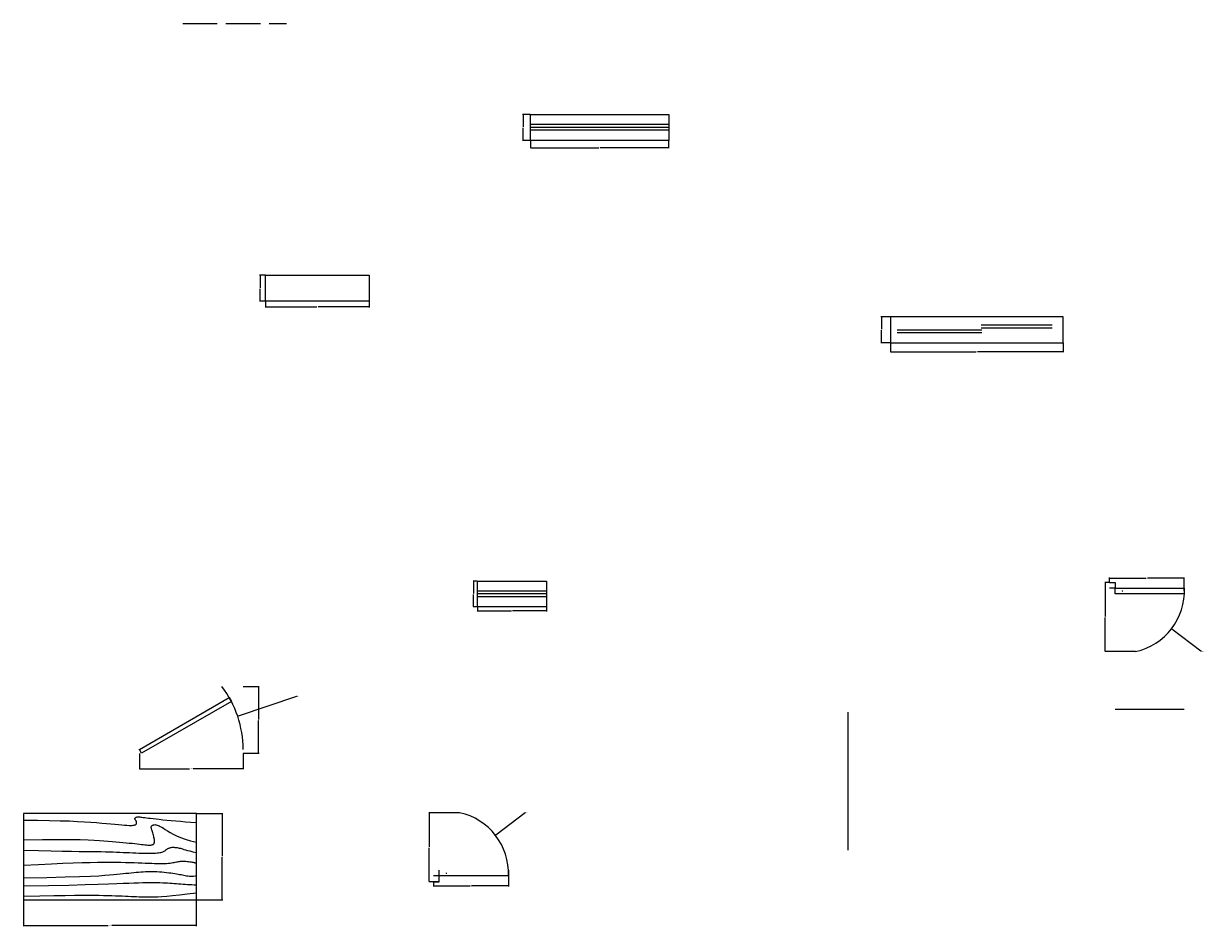
# Model space of a CAD drawing. Units: inches. Extents: x 821 to 2399, y 74 to 823.
# Tile 13 of 13: x 1989 to 2399, y 509 to 823. Entities that reach past the tile are written whole.
import ezdxf

# ---------------------------------------------------------------- set-up
doc = ezdxf.new("R2010")
doc.units = ezdxf.units.IN
doc.header["$MEASUREMENT"] = 0
doc.linetypes.add('ACAD_ISO02W100', pattern=[15, 12, -3])
doc.layers.get('0').update_dxf_attribs({"lineweight": 53})
for name, color, linetype, lineweight in [('A-ANNO-DIMS', 2, 'Continuous', 18), ('A-DOOR', 4, 'Continuous', 25), ('A-FURN', 8, 'Continuous', 18), ('A-GLAZ', 4, 'Continuous', 18), ('A-WALL-OVHD', 8, 'ACAD_ISO02W100', 18)]:
    doc.layers.add(name, color=color, linetype=linetype, lineweight=lineweight)
doc.styles.get("Standard").update_dxf_attribs({"font": 'arial.ttf'})
doc.dimstyles.get("Standard").update_dxf_attribs({"dimtxt": 0.18, "dimasz": 0.18, "dimexe": 0.18, "dimexo": 0.0625, "dimgap": 0.09, "dimtad": 0, "dimtih": 1, "dimtoh": 1, "dimdec": 4, "dimzin": 0, "dimdsep": 46, "dimtxsty": 'Standard', "dimcen": 0.09, "dimadec": 0, "dimazin": 0, "dimtfac": 1, "dimtdec": 4, "dimtofl": 0, "dimtmove": 0, "dimatfit": 3, "dimfxl": 1, "dimtolj": 1, "dimtzin": 0, "dimarcsym": 0})

# ---------------------------------------------------------------- blocks, each defined once
blk = doc.blocks.new('Table - Rectangular Woodgrain 60 x 30 in.')
for p, q in [((0, 0), (0, -30)), ((60, 0), (0, 0)), ((60, -30), (60, 0)), ((0, -30), (60, -30))]:
    blk.add_line(p, q)
for points in [[(0, -2.4), (4.8155, -2.418), (9.0302, -2.4688), (12.709, -2.5477), (15.9167, -2.65), (18.7181, -2.7711), (21.1781, -2.9063), (23.3616, -3.0508), (25.3333, -3.2), (27.1477, -3.3495), (28.8172, -3.4958), (30.3437, -3.636), (31.7291, -3.7667), (32.9756, -3.8849), (34.0849, -3.9875), (35.059, -4.0714), (35.9, -4.1334), (36.6114, -4.1711), (37.2041, -4.1854), (37.6906, -4.1779), (38.0833, -4.15), (38.3948, -4.1034), (38.6375, -4.0396), (38.8239, -3.9602), (38.9666, -3.8667), (39.0764, -3.7608), (39.1573, -3.6448), (39.2116, -3.521), (39.2416, -3.3917), (39.2498, -3.2593), (39.2385, -3.1261), (39.21, -2.9944), (39.1666, -2.8667), (39.111, -2.7447), (39.0468, -2.6281), (38.978, -2.5163), (38.9083, -2.4083), (38.8418, -2.3035), (38.7823, -2.201), (38.7337, -2.1001), (38.7, -2), (38.6844, -1.9003), (38.6875, -1.8021), (38.7094, -1.707), (38.75, -1.6167), (38.8094, -1.5326), (38.8875, -1.4563), (38.9844, -1.3893), (39.1, -1.3333), (39.2351, -1.2896), (39.3937, -1.2583), (39.5804, -1.2396), (39.8, -1.2333), (40.057, -1.2396), (40.3562, -1.2583), (40.7023, -1.2896), (41.1, -1.3333), (41.5547, -1.3895), (42.0755, -1.4573), (42.6721, -1.5361), (43.3542, -1.625), (44.1316, -1.7233), (45.014, -1.8302), (46.0114, -1.9449), (47.1333, -2.0667), (48.3862, -2.1947), (49.7625, -2.3281), (51.2513, -2.4663), (52.8416, -2.6083), (54.5226, -2.7535), (56.2833, -2.9011), (58.1127, -3.0501), (60, -3.2)], [(0, -9.2), (6.5759, -9.0858), (11.9385, -9.0365), (16.2527, -9.0418), (19.6833, -9.0917), (22.3952, -9.1759), (24.5531, -9.2844), (26.322, -9.4069), (27.8666, -9.5333), (29.3241, -9.6553), (30.7203, -9.7719), (32.0532, -9.8837), (33.3208, -9.9917), (34.5213, -10.0965), (35.6526, -10.199), (36.7128, -10.2999), (37.7, -10.4), (38.6129, -10.4996), (39.4531, -10.5969), (40.223, -10.6895), (40.925, -10.775), (41.5613, -10.8512), (42.1344, -10.9156), (42.6465, -10.966), (43.1, -11), (43.4976, -11.0158), (43.8437, -11.0136), (44.143, -10.9942), (44.4, -10.9583), (44.6195, -10.9069), (44.8062, -10.8406), (44.9648, -10.7603), (45.1, -10.6667), (45.2155, -10.5598), (45.3114, -10.4365), (45.3871, -10.2929), (45.4416, -10.125), (45.4743, -9.929), (45.4844, -9.7011), (45.4709, -9.4371), (45.4333, -9.1333), (45.3716, -8.7883), (45.2896, -8.4104), (45.1919, -8.0107), (45.0833, -7.6), (44.9685, -7.1893), (44.8521, -6.7896), (44.7388, -6.4117), (44.6333, -6.0667), (44.54, -5.7628), (44.4614, -5.4979), (44.4001, -5.2675), (44.3583, -5.0667), (44.3384, -4.8909), (44.3427, -4.7354), (44.3736, -4.5956), (44.4333, -4.4667), (44.5236, -4.3453), (44.6427, -4.2333), (44.7884, -4.1339), (44.9583, -4.05), (45.1501, -3.9849), (45.3614, -3.9417), (45.59, -3.9234), (45.8333, -3.9333), (46.0915, -3.9749), (46.3734, -4.0531), (46.6906, -4.1736), (47.0542, -4.3417), (47.4756, -4.5629), (47.9661, -4.8427), (48.5372, -5.1866), (49.2, -5.6), (49.9676, -6.0844), (50.8594, -6.625), (51.8965, -7.2031), (53.1, -7.8), (54.491, -8.3969), (56.0906, -8.975), (57.9199, -9.5156), (60, -10)], [(0, -12.8), (5.1847, -12.9322), (9.6213, -13.0323), (13.3963, -13.1059), (16.5958, -13.1583), (19.3063, -13.1952), (21.614, -13.2219), (23.6054, -13.2439), (25.3666, -13.2667), (26.9728, -13.2947), (28.4531, -13.3281), (29.8256, -13.3663), (31.1083, -13.4083), (32.3191, -13.4535), (33.476, -13.501), (34.597, -13.5501), (35.7, -13.6), (36.7984, -13.6497), (37.8875, -13.6979), (38.9578, -13.743), (40, -13.7833), (41.0047, -13.8174), (41.9625, -13.8438), (42.864, -13.8607), (43.7, -13.8667), (44.4631, -13.8604), (45.1552, -13.8417), (45.7801, -13.8104), (46.3416, -13.7667), (46.8439, -13.7104), (47.2906, -13.6417), (47.6858, -13.5604), (48.0333, -13.4667), (48.3375, -13.3608), (48.6042, -13.2448), (48.8396, -13.121), (49.05, -12.9917), (49.2417, -12.8593), (49.4208, -12.7261), (49.5937, -12.5944), (49.7667, -12.4667), (49.9452, -12.3451), (50.1323, -12.2313), (50.3303, -12.1268), (50.5416, -12.0333), (50.7686, -11.9524), (51.0135, -11.8854), (51.2788, -11.8341), (51.5666, -11.8), (51.8785, -11.7843), (52.2116, -11.7865), (52.562, -11.8059), (52.926, -11.8417), (53.2998, -11.8931), (53.6795, -11.9594), (54.0614, -12.0397), (54.4416, -12.1333), (54.8223, -12.2401), (55.2293, -12.3625), (55.6942, -12.5037), (56.2489, -12.6667), (56.9251, -12.8547), (57.7545, -13.0708), (58.7689, -13.3182), (60, -13.6)], [(0, -18), (5.124, -17.7273), (9.6609, -17.5057), (13.6705, -17.3303), (17.2125, -17.1958), (20.3467, -17.0973), (23.1328, -17.0297), (25.6307, -16.9878), (27.9, -16.9667), (29.9928, -16.9617), (31.9302, -16.9703), (33.7254, -16.9907), (35.3917, -17.0208), (36.9423, -17.0588), (38.3906, -17.1026), (39.7499, -17.1503), (41.0333, -17.2), (42.2519, -17.2496), (43.4073, -17.2969), (44.4986, -17.3395), (45.525, -17.375), (46.4858, -17.4012), (47.3802, -17.4156), (48.2074, -17.416), (48.9667, -17.4), (49.6583, -17.3662), (50.2872, -17.3167), (50.8595, -17.2547), (51.3812, -17.1833), (51.8584, -17.1057), (52.2971, -17.025), (52.7034, -16.9443), (53.0833, -16.8667), (53.443, -16.7951), (53.789, -16.7313), (54.128, -16.6768), (54.4666, -16.6334), (54.8115, -16.6024), (55.1693, -16.5854), (55.5465, -16.5841), (55.95, -16.6), (56.3828, -16.6337), (56.8346, -16.6823), (57.2915, -16.7418), (57.7396, -16.8084), (58.165, -16.878), (58.5539, -16.9469), (58.8924, -17.0111), (59.1666, -17.0667), (59.3679, -17.1107), (59.5078, -17.1438), (59.6032, -17.1675), (59.6708, -17.1833), (59.7275, -17.193), (59.7901, -17.1979), (59.8753, -17.1998), (60, -17.2)], [(0, -22.4), (8.0098, -22.2501), (14.4094, -22.1011), (19.4168, -21.9535), (23.25, -21.8083), (26.1269, -21.6663), (28.2656, -21.5281), (29.884, -21.3947), (31.2, -21.2667), (32.3967, -21.1448), (33.5172, -21.0292), (34.5697, -20.9198), (35.5625, -20.8167), (36.5037, -20.7198), (37.4015, -20.6292), (38.2642, -20.5448), (39.1, -20.4667), (39.9164, -20.3951), (40.7187, -20.3313), (41.5117, -20.2768), (42.3, -20.2333), (43.0883, -20.2024), (43.8812, -20.1854), (44.6836, -20.1841), (45.5, -20.2), (46.3328, -20.234), (47.1747, -20.2844), (48.0163, -20.3488), (48.8479, -20.425), (49.66, -20.5106), (50.4429, -20.6031), (51.1872, -20.7004), (51.8833, -20.8), (52.5246, -20.8999), (53.1166, -20.9995), (53.6681, -21.0983), (54.1875, -21.1958), (54.6834, -21.2919), (55.1646, -21.3859), (55.6394, -21.4777), (56.1167, -21.5667), (56.6028, -21.6515), (57.0961, -21.7266), (57.5929, -21.7852), (58.0896, -21.8208), (58.5823, -21.8268), (59.0674, -21.7964), (59.5412, -21.723), (60, -21.6)], [(0, -25.2), (8.6355, -25.0504), (15.7026, -24.9031), (21.4049, -24.7606), (25.9458, -24.625), (29.529, -24.4988), (32.3578, -24.3844), (34.6359, -24.284), (36.5667, -24.2), (38.3213, -24.1341), (39.9417, -24.0854), (41.437, -24.0523), (42.8167, -24.0333), (44.0901, -24.0268), (45.2667, -24.0313), (46.3557, -24.0451), (47.3667, -24.0667), (48.309, -24.0947), (49.1928, -24.1287), (50.0284, -24.168), (50.826, -24.2125), (51.5959, -24.2617), (52.3483, -24.3151), (53.0935, -24.3725), (53.8417, -24.4334), (54.6009, -24.497), (55.3699, -24.561), (56.1454, -24.6226), (56.9239, -24.6792), (57.7021, -24.7279), (58.4764, -24.7662), (59.2435, -24.7911), (60, -24.8)], [(0, -28.8), (5.6867, -28.6681), (10.45, -28.5698), (14.407, -28.5012), (17.675, -28.4584), (20.3711, -28.4374), (22.6125, -28.4344), (24.5164, -28.4455), (26.2, -28.4667), (27.762, -28.4947), (29.2276, -28.5281), (30.6033, -28.5663), (31.8958, -28.6084), (33.1118, -28.6535), (34.2578, -28.7011), (35.3405, -28.7501), (36.3666, -28.8), (37.3443, -28.8497), (38.288, -28.8974), (39.2137, -28.9412), (40.1375, -28.9792), (41.0753, -29.0093), (42.0432, -29.0297), (43.0572, -29.0384), (44.1333, -29.0333), (45.2936, -29.0114), (46.5843, -28.9641), (48.0579, -28.8816), (49.7666, -28.7542), (51.7629, -28.5721), (54.0989, -28.3255), (56.8272, -28.0048), (60, -27.6)]]:
    blk.add_lwpolyline(points)
blk = doc.blocks.new('Door - Left Hung 36 in.')
blk.add_lwpolyline([(0.75, -1.3), (0, 0), (31.18, 18), (31.93, 16.7)], close=True)
blk.add_arc((0, 0), 36, 0, 37.3101)
blk = doc.blocks.new('*D68')
at = {"layer": 'A-ANNO-DIMS', "color": 0, "lineweight": -2, "transparency": 16777216}
for p, q in [((1989.31, 518.7), (1989.31, 509.59)), ((2049.31, 518.7), (2049.31, 509.59)), ((1989.49, 509.77), (2018.66, 509.77)), ((2049.13, 509.77), (2019.97, 509.77))]:
    blk.add_line(p, q, dxfattribs=at)
at = {"layer": 'A-ANNO-DIMS', "color": 0, "lineweight": 50, "transparency": 16777216}
for points in [[(1989.49, 509.8), (1989.49, 509.74), (1989.31, 509.77)], [(2049.13, 509.8), (2049.13, 509.74), (2049.31, 509.77)]]:
    blk.add_solid(points, dxfattribs=at)
at = {"layer": 'Defpoints', "color": 0, "lineweight": 50, "transparency": 16777216}
for p in [(1989.31, 518.77), (2049.31, 518.77), (2049.31, 509.77)]:
    blk.add_point(p, dxfattribs=at)
at = {"layer": 'A-ANNO-DIMS', "color": 0, "transparency": 16777216, "insert": (2019.31, 509.77), "char_height": 0.18, "attachment_point": 5}
blk.add_mtext('\\A1;TABLE 60', dxfattribs=at)
blk = doc.blocks.new('*D69')
at = {"layer": 'A-ANNO-DIMS', "color": 0, "lineweight": -2, "transparency": 16777216}
for p, q in [((2049.37, 548.77), (2058.49, 548.77)), ((2058.31, 548.59), (2058.31, 533.95)), ((2058.31, 518.95), (2058.31, 533.58)), ((2049.37, 518.77), (2058.49, 518.77))]:
    blk.add_line(p, q, dxfattribs=at)
at = {"layer": 'A-ANNO-DIMS', "color": 0, "lineweight": 50, "transparency": 16777216}
for points in [[(2058.28, 548.59), (2058.34, 548.59), (2058.31, 548.77)], [(2058.28, 518.95), (2058.34, 518.95), (2058.31, 518.77)]]:
    blk.add_solid(points, dxfattribs=at)
at = {"layer": 'Defpoints', "color": 0, "lineweight": 50, "transparency": 16777216}
for p in [(2049.31, 548.77), (2058.31, 548.77), (2049.31, 518.77)]:
    blk.add_point(p, dxfattribs=at)
at = {"layer": 'A-ANNO-DIMS', "color": 0, "transparency": 16777216, "insert": (2058.31, 533.77), "char_height": 0.18, "attachment_point": 5}
blk.add_mtext('\\A1;30', dxfattribs=at)
blk = doc.blocks.new('*D74')
at = {"layer": 'A-ANNO-DIMS', "color": 0, "lineweight": -2, "transparency": 16777216}
for p, q in [((2029.56, 569.62), (2029.56, 564.1)), ((2065.56, 569.62), (2065.56, 564.1)), ((2029.74, 564.28), (2046.94, 564.28)), ((2065.38, 564.28), (2048.19, 564.28))]:
    blk.add_line(p, q, dxfattribs=at)
at = {"layer": 'A-ANNO-DIMS', "color": 0, "lineweight": 50, "transparency": 16777216}
for points in [[(2029.74, 564.31), (2029.74, 564.25), (2029.56, 564.28)], [(2065.38, 564.31), (2065.38, 564.25), (2065.56, 564.28)]]:
    blk.add_solid(points, dxfattribs=at)
at = {"layer": 'Defpoints', "color": 0, "lineweight": 50, "transparency": 16777216}
for p in [(2029.56, 569.68), (2065.56, 569.68), (2065.56, 564.28)]:
    blk.add_point(p, dxfattribs=at)
at = {"layer": 'A-ANNO-DIMS', "color": 0, "transparency": 16777216, "insert": (2047.56, 564.28), "char_height": 0.18, "attachment_point": 5}
blk.add_mtext('\\A1;DOOR 36', dxfattribs=at)
blk = doc.blocks.new('*D75')
at = {"layer": 'A-ANNO-DIMS', "color": 0, "lineweight": -2, "transparency": 16777216}
for p, q in [((2065.63, 592.8), (2071.14, 592.8)), ((2070.96, 592.62), (2070.96, 581.42)), ((2070.96, 569.86), (2070.96, 581.06)), ((2065.63, 569.68), (2071.14, 569.68))]:
    blk.add_line(p, q, dxfattribs=at)
at = {"layer": 'A-ANNO-DIMS', "color": 0, "lineweight": 50, "transparency": 16777216}
for points in [[(2070.93, 592.62), (2070.99, 592.62), (2070.96, 592.8)], [(2070.93, 569.86), (2070.99, 569.86), (2070.96, 569.68)]]:
    blk.add_solid(points, dxfattribs=at)
at = {"layer": 'Defpoints', "color": 0, "lineweight": 50, "transparency": 16777216}
for p in [(2065.56, 592.8), (2070.96, 592.8), (2065.56, 569.68)]:
    blk.add_point(p, dxfattribs=at)
at = {"layer": 'A-ANNO-DIMS', "color": 0, "transparency": 16777216, "insert": (2070.96, 581.24), "char_height": 0.18, "attachment_point": 5}
blk.add_mtext('\\A1;23', dxfattribs=at)
blk = doc.blocks.new('*D120')
at = {"layer": 'A-ANNO-DIMS', "color": 0, "lineweight": -2, "transparency": 16777216}
for p, q in [((2165.39, 782.53), (2165.39, 779.86)), ((2165.57, 780.04), (2189.17, 780.04)), ((2213.21, 780.04), (2189.62, 780.04)), ((2213.39, 782.53), (2213.39, 779.86))]:
    blk.add_line(p, q, dxfattribs=at)
at = {"layer": 'A-ANNO-DIMS', "color": 0, "lineweight": 50, "transparency": 16777216}
for points in [[(2165.57, 780.07), (2165.57, 780.01), (2165.39, 780.04)], [(2213.21, 780.07), (2213.21, 780.01), (2213.39, 780.04)]]:
    blk.add_solid(points, dxfattribs=at)
at = {"layer": 'Defpoints', "color": 0, "lineweight": 50, "transparency": 16777216}
for p in [(2165.39, 782.59), (2213.39, 782.59), (2213.39, 780.04)]:
    blk.add_point(p, dxfattribs=at)
at = {"layer": 'A-ANNO-DIMS', "color": 0, "transparency": 16777216, "insert": (2189.39, 780.04), "char_height": 0.18, "attachment_point": 5}
blk.add_mtext('\\A1;48', dxfattribs=at)
blk = doc.blocks.new('*D121')
at = {"layer": 'A-ANNO-DIMS', "color": 0, "lineweight": -2, "transparency": 16777216}
for p, q in [((2165.33, 791.59), (2162.66, 791.59)), ((2162.84, 791.41), (2162.84, 787.27)), ((2162.84, 782.77), (2162.84, 786.91)), ((2165.33, 782.59), (2162.66, 782.59))]:
    blk.add_line(p, q, dxfattribs=at)
at = {"layer": 'A-ANNO-DIMS', "color": 0, "lineweight": 50, "transparency": 16777216}
for points in [[(2162.81, 791.41), (2162.87, 791.41), (2162.84, 791.59)], [(2162.81, 782.77), (2162.87, 782.77), (2162.84, 782.59)]]:
    blk.add_solid(points, dxfattribs=at)
at = {"layer": 'Defpoints', "color": 0, "lineweight": 50, "transparency": 16777216}
for p in [(2162.84, 791.59), (2165.39, 791.59), (2165.39, 782.59)]:
    blk.add_point(p, dxfattribs=at)
at = {"layer": 'A-ANNO-DIMS', "color": 0, "transparency": 16777216, "insert": (2162.84, 787.09), "char_height": 0.18, "attachment_point": 5}
blk.add_mtext('\\A1;9', dxfattribs=at)
blk = doc.blocks.new('*D122')
at = {"layer": 'A-ANNO-DIMS', "color": 0, "lineweight": -2, "transparency": 16777216}
for p, q in [((2146.98, 620.43), (2146.98, 618.96)), ((2170.98, 620.43), (2170.98, 618.96)), ((2147.16, 619.14), (2158.76, 619.14)), ((2170.8, 619.14), (2159.2, 619.14))]:
    blk.add_line(p, q, dxfattribs=at)
at = {"layer": 'A-ANNO-DIMS', "color": 0, "lineweight": 50, "transparency": 16777216}
for points in [[(2147.16, 619.17), (2147.16, 619.11), (2146.98, 619.14)], [(2170.8, 619.17), (2170.8, 619.11), (2170.98, 619.14)]]:
    blk.add_solid(points, dxfattribs=at)
at = {"layer": 'Defpoints', "color": 0, "lineweight": 50, "transparency": 16777216}
for p in [(2146.98, 620.49), (2170.98, 620.49), (2170.98, 619.14)]:
    blk.add_point(p, dxfattribs=at)
at = {"layer": 'A-ANNO-DIMS', "color": 0, "transparency": 16777216, "insert": (2158.98, 619.14), "char_height": 0.18, "attachment_point": 5}
blk.add_mtext('\\A1;24', dxfattribs=at)
blk = doc.blocks.new('*D123')
at = {"layer": 'A-ANNO-DIMS', "color": 0, "lineweight": -2, "transparency": 16777216}
for p, q in [((2146.92, 629.49), (2145.45, 629.49)), ((2145.63, 629.31), (2145.63, 625.17)), ((2145.63, 620.67), (2145.63, 624.81)), ((2146.92, 620.49), (2145.45, 620.49))]:
    blk.add_line(p, q, dxfattribs=at)
at = {"layer": 'A-ANNO-DIMS', "color": 0, "lineweight": 50, "transparency": 16777216}
for points in [[(2145.6, 629.31), (2145.66, 629.31), (2145.63, 629.49)], [(2145.6, 620.67), (2145.66, 620.67), (2145.63, 620.49)]]:
    blk.add_solid(points, dxfattribs=at)
at = {"layer": 'Defpoints', "color": 0, "lineweight": 50, "transparency": 16777216}
for p in [(2145.63, 629.49), (2146.98, 629.49), (2146.98, 620.49)]:
    blk.add_point(p, dxfattribs=at)
at = {"layer": 'A-ANNO-DIMS', "color": 0, "transparency": 16777216, "insert": (2145.63, 624.99), "char_height": 0.18, "attachment_point": 5}
blk.add_mtext('\\A1;9', dxfattribs=at)
blk = doc.blocks.new('*D124')
at = {"layer": 'A-ANNO-DIMS', "color": 0, "lineweight": -2, "transparency": 16777216}
for p, q in [((2073.39, 726.65), (2073.39, 724.58)), ((2109.39, 726.65), (2109.39, 724.58)), ((2073.57, 724.76), (2091.17, 724.76)), ((2109.21, 724.76), (2091.6, 724.76))]:
    blk.add_line(p, q, dxfattribs=at)
at = {"layer": 'A-ANNO-DIMS', "color": 0, "lineweight": 50, "transparency": 16777216}
for points in [[(2073.57, 724.79), (2073.57, 724.73), (2073.39, 724.76)], [(2109.21, 724.79), (2109.21, 724.73), (2109.39, 724.76)]]:
    blk.add_solid(points, dxfattribs=at)
at = {"layer": 'Defpoints', "color": 0, "lineweight": 50, "transparency": 16777216}
for p in [(2073.39, 726.71), (2109.39, 726.71), (2109.39, 724.76)]:
    blk.add_point(p, dxfattribs=at)
at = {"layer": 'A-ANNO-DIMS', "color": 0, "transparency": 16777216, "insert": (2091.39, 724.76), "char_height": 0.18, "attachment_point": 5}
blk.add_mtext('\\A1;36', dxfattribs=at)
blk = doc.blocks.new('*D125')
at = {"layer": 'A-ANNO-DIMS', "color": 0, "lineweight": -2, "transparency": 16777216}
for p, q in [((2073.32, 735.71), (2071.26, 735.71)), ((2071.44, 735.53), (2071.44, 731.39)), ((2071.44, 726.89), (2071.44, 731.03)), ((2073.32, 726.71), (2071.26, 726.71))]:
    blk.add_line(p, q, dxfattribs=at)
at = {"layer": 'A-ANNO-DIMS', "color": 0, "lineweight": 50, "transparency": 16777216}
for points in [[(2071.41, 735.53), (2071.47, 735.53), (2071.44, 735.71)], [(2071.41, 726.89), (2071.47, 726.89), (2071.44, 726.71)]]:
    blk.add_solid(points, dxfattribs=at)
at = {"layer": 'Defpoints', "color": 0, "lineweight": 50, "transparency": 16777216}
for p in [(2071.44, 735.71), (2073.39, 735.71), (2073.39, 726.71)]:
    blk.add_point(p, dxfattribs=at)
at = {"layer": 'A-ANNO-DIMS', "color": 0, "transparency": 16777216, "insert": (2071.44, 731.21), "char_height": 0.18, "attachment_point": 5}
blk.add_mtext('\\A1;9', dxfattribs=at)
blk = doc.blocks.new('*D126')
at = {"layer": 'A-ANNO-DIMS', "color": 0, "lineweight": -2, "transparency": 16777216}
for p, q in [((2290.44, 712.24), (2290.44, 708.97)), ((2350.44, 712.24), (2350.44, 708.97)), ((2290.62, 709.15), (2320.22, 709.15)), ((2350.26, 709.15), (2320.66, 709.15))]:
    blk.add_line(p, q, dxfattribs=at)
at = {"layer": 'A-ANNO-DIMS', "color": 0, "lineweight": 50, "transparency": 16777216}
for points in [[(2290.62, 709.18), (2290.62, 709.12), (2290.44, 709.15)], [(2350.26, 709.18), (2350.26, 709.12), (2350.44, 709.15)]]:
    blk.add_solid(points, dxfattribs=at)
at = {"layer": 'Defpoints', "color": 0, "lineweight": 50, "transparency": 16777216}
for p in [(2290.44, 712.3), (2350.44, 712.3), (2350.44, 709.15)]:
    blk.add_point(p, dxfattribs=at)
at = {"layer": 'A-ANNO-DIMS', "color": 0, "transparency": 16777216, "insert": (2320.44, 709.15), "char_height": 0.18, "attachment_point": 5}
blk.add_mtext('\\A1;60', dxfattribs=at)
blk = doc.blocks.new('*D127')
at = {"layer": 'A-ANNO-DIMS', "color": 0, "lineweight": -2, "transparency": 16777216}
for p, q in [((2290.38, 721.3), (2287.11, 721.3)), ((2287.29, 721.12), (2287.29, 716.98)), ((2287.29, 712.48), (2287.29, 716.62)), ((2290.38, 712.3), (2287.11, 712.3))]:
    blk.add_line(p, q, dxfattribs=at)
at = {"layer": 'A-ANNO-DIMS', "color": 0, "lineweight": 50, "transparency": 16777216}
for points in [[(2287.26, 721.12), (2287.32, 721.12), (2287.29, 721.3)], [(2287.26, 712.48), (2287.32, 712.48), (2287.29, 712.3)]]:
    blk.add_solid(points, dxfattribs=at)
at = {"layer": 'Defpoints', "color": 0, "lineweight": 50, "transparency": 16777216}
for p in [(2287.29, 721.3), (2290.44, 721.3), (2290.44, 712.3)]:
    blk.add_point(p, dxfattribs=at)
at = {"layer": 'A-ANNO-DIMS', "color": 0, "transparency": 16777216, "insert": (2287.29, 716.8), "char_height": 0.18, "attachment_point": 5}
blk.add_mtext('\\A1;9', dxfattribs=at)
blk = doc.blocks.new('*D130')
at = {"layer": 'A-ANNO-DIMS', "color": 0, "lineweight": -2, "transparency": 16777216}
for p, q in [((2157.7, 526.95), (2157.7, 523.38)), ((2131.7, 524.95), (2131.7, 523.38)), ((2131.88, 523.56), (2144.48, 523.56)), ((2157.52, 523.56), (2144.92, 523.56))]:
    blk.add_line(p, q, dxfattribs=at)
at = {"layer": 'A-ANNO-DIMS', "color": 0, "lineweight": 50, "transparency": 16777216}
for points in [[(2131.88, 523.59), (2131.88, 523.53), (2131.7, 523.56)], [(2157.52, 523.59), (2157.52, 523.53), (2157.7, 523.56)]]:
    blk.add_solid(points, dxfattribs=at)
at = {"layer": 'Defpoints', "color": 0, "lineweight": 50, "transparency": 16777216}
for p in [(2157.7, 527.01), (2131.7, 525.01), (2157.7, 523.56)]:
    blk.add_point(p, dxfattribs=at)
at = {"layer": 'A-ANNO-DIMS', "color": 0, "transparency": 16777216, "insert": (2144.7, 523.56), "char_height": 0.18, "attachment_point": 5}
blk.add_mtext('\\A1;26', dxfattribs=at)
blk = doc.blocks.new('*D131')
at = {"layer": 'A-ANNO-DIMS', "color": 0, "lineweight": -2, "transparency": 16777216}
for p, q in [((2140.71, 549.01), (2130.07, 549.01)), ((2130.25, 548.83), (2130.25, 537.19)), ((2130.25, 525.19), (2130.25, 536.83)), ((2133.64, 525.01), (2130.07, 525.01))]:
    blk.add_line(p, q, dxfattribs=at)
at = {"layer": 'A-ANNO-DIMS', "color": 0, "lineweight": 50, "transparency": 16777216}
for points in [[(2130.22, 548.83), (2130.28, 548.83), (2130.25, 549.01)], [(2130.22, 525.19), (2130.28, 525.19), (2130.25, 525.01)]]:
    blk.add_solid(points, dxfattribs=at)
at = {"layer": 'Defpoints', "color": 0, "lineweight": 50, "transparency": 16777216}
for p in [(2130.25, 549.01), (2140.78, 549.01), (2133.7, 525.01)]:
    blk.add_point(p, dxfattribs=at)
at = {"layer": 'A-ANNO-DIMS', "color": 0, "transparency": 16777216, "insert": (2130.25, 537.01), "char_height": 0.18, "attachment_point": 5}
blk.add_mtext('\\A1;24', dxfattribs=at)
blk = doc.blocks.new('*D132')
at = {"layer": 'A-ANNO-DIMS', "color": 0, "lineweight": -2, "transparency": 16777216}
for p, q in [((2366.52, 629.09), (2366.52, 630.68)), ((2366.7, 630.5), (2379.3, 630.5)), ((2392.34, 630.5), (2379.74, 630.5)), ((2392.52, 627.09), (2392.52, 630.68))]:
    blk.add_line(p, q, dxfattribs=at)
at = {"layer": 'A-ANNO-DIMS', "color": 0, "lineweight": 50, "transparency": 16777216}
for points in [[(2366.7, 630.53), (2366.7, 630.47), (2366.52, 630.5)], [(2392.34, 630.53), (2392.34, 630.47), (2392.52, 630.5)]]:
    blk.add_solid(points, dxfattribs=at)
at = {"layer": 'Defpoints', "color": 0, "lineweight": 50, "transparency": 16777216}
for p in [(2366.52, 629.03), (2392.52, 630.5), (2392.52, 627.03)]:
    blk.add_point(p, dxfattribs=at)
at = {"layer": 'A-ANNO-DIMS', "color": 0, "transparency": 16777216, "insert": (2379.52, 630.5), "char_height": 0.18, "attachment_point": 5}
blk.add_mtext('\\A1;26', dxfattribs=at)
blk = doc.blocks.new('*D133')
at = {"layer": 'A-ANNO-DIMS', "color": 0, "lineweight": -2, "transparency": 16777216}
for p, q in [((2366.46, 629.03), (2364.87, 629.03)), ((2365.05, 628.85), (2365.05, 617.21)), ((2365.05, 605.21), (2365.05, 616.85)), ((2375.54, 605.03), (2364.87, 605.03))]:
    blk.add_line(p, q, dxfattribs=at)
at = {"layer": 'A-ANNO-DIMS', "color": 0, "lineweight": 50, "transparency": 16777216}
for points in [[(2365.02, 628.85), (2365.08, 628.85), (2365.05, 629.03)], [(2365.02, 605.21), (2365.08, 605.21), (2365.05, 605.03)]]:
    blk.add_solid(points, dxfattribs=at)
at = {"layer": 'Defpoints', "color": 0, "lineweight": 50, "transparency": 16777216}
for p in [(2366.52, 629.03), (2365.05, 605.03), (2375.6, 605.03)]:
    blk.add_point(p, dxfattribs=at)
at = {"layer": 'A-ANNO-DIMS', "color": 0, "transparency": 16777216, "insert": (2365.05, 617.03), "char_height": 0.18, "attachment_point": 5}
blk.add_mtext('\\A1;24', dxfattribs=at)
blk = doc.blocks.new('*D151')
at = {"layer": 'A-ANNO-DIMS', "color": 0, "lineweight": -2, "transparency": 16777216}
for p, q in [((2163.49, 548.97), (2153.41, 541.22)), ((2163.67, 548.97), (2163.49, 548.97)), ((2136.15, 528.01), (2136.33, 528.01)), ((2136.24, 527.92), (2136.24, 528.1))]:
    blk.add_line(p, q, dxfattribs=at)
at = {"layer": 'A-ANNO-DIMS', "color": 0, "lineweight": 50, "transparency": 16777216}
blk.add_solid([(2153.39, 541.24), (2153.43, 541.19), (2153.27, 541.11)], dxfattribs=at)
at = {"layer": 'Defpoints', "color": 0, "lineweight": 50, "transparency": 16777216}
for p in [(2153.27, 541.11), (2136.24, 528.01)]:
    blk.add_point(p, dxfattribs=at)
at = {"layer": 'A-ANNO-DIMS', "color": 0, "transparency": 16777216, "insert": (2164.22, 548.97), "char_height": 0.18, "attachment_point": 5}
blk.add_mtext('\\A1;R21.485', dxfattribs=at)
blk = doc.blocks.new('*D152')
at = {"layer": 'A-ANNO-DIMS', "color": 0, "lineweight": -2, "transparency": 16777216}
for p, q in [((2370.97, 626.03), (2371.15, 626.03)), ((2371.06, 625.94), (2371.06, 626.12)), ((2398.31, 605.07), (2388.23, 612.82)), ((2398.49, 605.07), (2398.31, 605.07))]:
    blk.add_line(p, q, dxfattribs=at)
at = {"layer": 'A-ANNO-DIMS', "color": 0, "lineweight": 50, "transparency": 16777216}
blk.add_solid([(2388.25, 612.84), (2388.22, 612.79), (2388.09, 612.93)], dxfattribs=at)
at = {"layer": 'Defpoints', "color": 0, "lineweight": 50, "transparency": 16777216}
for p in [(2371.06, 626.03), (2388.09, 612.93)]:
    blk.add_point(p, dxfattribs=at)
at = {"layer": 'A-ANNO-DIMS', "color": 0, "transparency": 16777216, "insert": (2399.04, 605.07), "char_height": 0.18, "attachment_point": 5}
blk.add_mtext('\\A1;R21.485', dxfattribs=at)
blk = doc.blocks.new('*D153')
at = {"layer": 'A-ANNO-DIMS', "color": 0, "lineweight": -2, "transparency": 16777216}
for p, q in [((2084.14, 589.4), (2063.84, 582.55)), ((2084.32, 589.4), (2084.14, 589.4)), ((2029.47, 570.98), (2029.65, 570.98)), ((2029.56, 570.89), (2029.56, 571.07))]:
    blk.add_line(p, q, dxfattribs=at)
at = {"layer": 'A-ANNO-DIMS', "color": 0, "lineweight": 50, "transparency": 16777216}
blk.add_solid([(2063.83, 582.58), (2063.85, 582.52), (2063.67, 582.49)], dxfattribs=at)
at = {"layer": 'Defpoints', "color": 0, "lineweight": 50, "transparency": 16777216}
for p in [(2063.67, 582.49), (2029.56, 570.98)]:
    blk.add_point(p, dxfattribs=at)
at = {"layer": 'A-ANNO-DIMS', "color": 0, "transparency": 16777216, "insert": (2084.62, 589.4), "char_height": 0.18, "attachment_point": 5}
blk.add_mtext('\\A1;R36', dxfattribs=at)

msp = doc.modelspace()

# ---------------------------------------------------------------- linework, layer by layer
at = {"layer": 'A-DOOR'}
for p, q in [((2350.4382, 721.3027), (2290.4382, 721.3027)), ((2290.4382, 721.3027), (2290.4382, 712.3027)), ((2321.9728, 718.4911), (2346.5566, 718.4911)), ((2350.4382, 712.3027), (2350.4382, 721.3027)), ((2292.8065, 716.8027), (2322.216, 716.8027)), ((2292.8065, 715.8027), (2322.216, 715.8027)), ((2321.9728, 717.4911), (2346.5566, 717.4911)), ((2290.4382, 712.3027), (2350.4382, 712.3027)), ((2366.5232, 629.0259), (2368.5232, 629.0259)), ((2368.5232, 629.0259), (2368.5232, 627.0259)), ((2368.5232, 627.0259), (2366.5232, 627.0259)), ((2368.5232, 627.0259), (2392.5232, 627.0259)), ((2368.5232, 625.0259), (2368.5232, 627.0259)), ((2392.5232, 625.0259), (2368.5232, 625.0259)), ((2392.5232, 627.0259), (2392.5232, 625.0259)), ((2275.5874, 583.9331), (2275.5874, 535.9331)), ((2368.5232, 585.0259), (2392.5232, 585.0259)), ((2133.7, 527.009), (2131.7, 527.009)), ((2133.7, 527.009), (2133.7, 529.009)), ((2133.7, 525.009), (2133.7, 527.009)), ((2157.7, 527.009), (2133.7, 527.009)), ((2157.7, 529.009), (2157.7, 527.009)), ((2131.7, 525.009), (2133.7, 525.009))]:
    msp.add_line(p, q, dxfattribs=at)
for centre, start, end in [((2371.0617, 626.0259), 282.19505, 2.667766), ((2136.2385, 528.009), 357.332234, 77.80495)]:
    msp.add_arc(centre, 21.4848, start, end, dxfattribs=at)
at = {"layer": 'A-GLAZ'}
for p, q in [((2165.3942, 782.5891), (2165.3942, 791.5891)), ((2165.3942, 791.5891), (2213.3942, 791.5891)), ((2213.3942, 788.0891), (2165.3942, 788.0891)), ((2213.3942, 791.5891), (2213.3942, 782.5891)), ((2213.3942, 787.0891), (2165.3942, 787.0891)), ((2213.3942, 786.0891), (2165.3942, 786.0891)), ((2213.3942, 782.5891), (2165.3942, 782.5891)), ((2073.3855, 735.709), (2109.3855, 735.709)), ((2073.3855, 726.709), (2073.3855, 735.709)), ((2109.3855, 735.709), (2109.3855, 726.709)), ((2109.3855, 726.709), (2073.3855, 726.709)), ((2146.9794, 629.4882), (2170.9794, 629.4882)), ((2146.9794, 620.4882), (2146.9794, 629.4882)), ((2170.9794, 629.4882), (2170.9794, 620.4882)), ((2170.9794, 625.9882), (2146.9794, 625.9882)), ((2170.9794, 624.9882), (2146.9794, 624.9882)), ((2170.9794, 623.9882), (2146.9794, 623.9882)), ((2170.9794, 620.4882), (2146.9794, 620.4882))]:
    msp.add_line(p, q, dxfattribs=at)
at = {"layer": 'A-WALL-OVHD'}
msp.add_line((2044.5892, 823.1645), (2080.5892, 823.1645), dxfattribs=at)

# ---------------------------------------------------------------- block references
at = {"layer": 'A-DOOR'}
msp.add_blockref('Door - Left Hung 36 in.', (2029.5649, 570.9778), dxfattribs=at)
at = {"layer": 'A-FURN'}
msp.add_blockref('Table - Rectangular Woodgrain 60 x 30 in.', (1989.3118, 548.7667), dxfattribs=at)

# ---------------------------------------------------------------- dimensions: what is measured, and where the dimension line sits
at = {"layer": 'A-ANNO-DIMS'}
for base, p1, p2, picture, middle in [((2162.8442, 791.5891), (2165.3942, 782.5891), (2165.3942, 791.5891), '*D121', (2162.8442, 787.0891)), ((2071.4355, 735.709), (2073.3855, 726.709), (2073.3855, 735.709), '*D125', (2071.4355, 731.209)), ((2287.2882, 721.3027), (2290.4382, 712.3027), (2290.4382, 721.3027), '*D127', (2287.2882, 716.8027)), ((2145.6294, 629.4882), (2146.9794, 620.4882), (2146.9794, 629.4882), '*D123', (2145.6294, 624.9882)), ((2365.0482, 605.0259), (2366.5232, 629.0259), (2375.6002, 605.0259), '*D133', (2365.0482, 617.0259)), ((2070.9649, 592.7985), (2065.5649, 569.6788), (2065.5649, 592.7985), '*D75', (2070.9649, 581.2386)), ((2058.3118, 548.7667), (2049.3118, 518.7667), (2049.3118, 548.7667), '*D69', (2058.3118, 533.7667)), ((2130.25, 549.009), (2133.7, 525.009), (2140.7769, 549.009), '*D131', (2130.25, 537.009))]:
    dim = msp.add_linear_dim(base=base, p1=p1, p2=p2, angle=90, dimstyle='Standard', override={"dimdec": 0, "dimlfac": 1, "dimrnd": 0, "dimzin": 0, "dimdsep": 46, "dimlunit": 2}, dxfattribs=at)
    dim.commit()
    dim.dimension.update_dxf_attribs({"geometry": picture, "text_midpoint": middle})
for base, p1, p2, picture, middle in [((2213.3942, 780.0391), (2165.3942, 782.5891), (2213.3942, 782.5891), '*D120', (2189.3942, 780.0391)), ((2109.3855, 724.759), (2073.3855, 726.709), (2109.3855, 726.709), '*D124', (2091.3855, 724.759)), ((2350.4382, 709.1527), (2290.4382, 712.3027), (2350.4382, 712.3027), '*D126', (2320.4382, 709.1527)), ((2392.5232, 630.5009), (2366.5232, 629.0259), (2392.5232, 627.0259), '*D132', (2379.5232, 630.5009)), ((2170.9794, 619.1382), (2146.9794, 620.4882), (2170.9794, 620.4882), '*D122', (2158.9794, 619.1382)), ((2157.7, 523.559), (2131.7, 525.009), (2157.7, 527.009), '*D130', (2144.7, 523.559))]:
    dim = msp.add_linear_dim(base=base, p1=p1, p2=p2, dimstyle='Standard', override={"dimdec": 0, "dimlfac": 1, "dimrnd": 0, "dimzin": 0, "dimdsep": 46, "dimlunit": 2}, dxfattribs=at)
    dim.commit()
    dim.dimension.update_dxf_attribs({"geometry": picture, "text_midpoint": middle})
for center, mpoint, override, picture, middle in [((2371.0617, 626.0259), (2388.0909, 612.9261), {"dimdec": 3, "dimlfac": 1, "dimrnd": 0, "dimzin": 0, "dimdsep": 46, "dimlunit": 2}, '*D152', (2399.0389, 605.0662)), ((2029.5649, 570.9778), (2063.6736, 582.4929), {"dimdec": 0, "dimlfac": 1, "dimrnd": 0, "dimzin": 0, "dimdsep": 46, "dimlunit": 2}, '*D153', (2084.6239, 589.4019)), ((2136.2385, 528.009), (2153.2677, 541.1088), {"dimdec": 3, "dimlfac": 1, "dimrnd": 0, "dimzin": 0, "dimdsep": 46, "dimlunit": 2}, '*D151', (2164.2157, 548.9686))]:
    dim = msp.add_radius_dim(center=center, mpoint=mpoint, dimstyle='Standard', override=override, dxfattribs=at)
    dim.commit()
    dim.dimension.update_dxf_attribs({"geometry": picture, "text_midpoint": middle, "dimtype": 164})
for base, p1, p2, text, picture, middle in [((2065.5649, 564.2788), (2029.5649, 569.6788), (2065.5649, 569.6788), 'DOOR <>', '*D74', (2047.5649, 564.2788)), ((2049.3118, 509.7667), (1989.3118, 518.7667), (2049.3118, 518.7667), 'TABLE <>', '*D68', (2019.3118, 509.7667))]:
    dim = msp.add_linear_dim(base=base, p1=p1, p2=p2, text=text, dimstyle='Standard', override={"dimdec": 0, "dimlfac": 1, "dimrnd": 0, "dimzin": 0, "dimdsep": 46, "dimlunit": 2}, dxfattribs=at)
    dim.commit()
    dim.dimension.update_dxf_attribs({"geometry": picture, "text_midpoint": middle})

doc.saveas('drawing.dxf')
